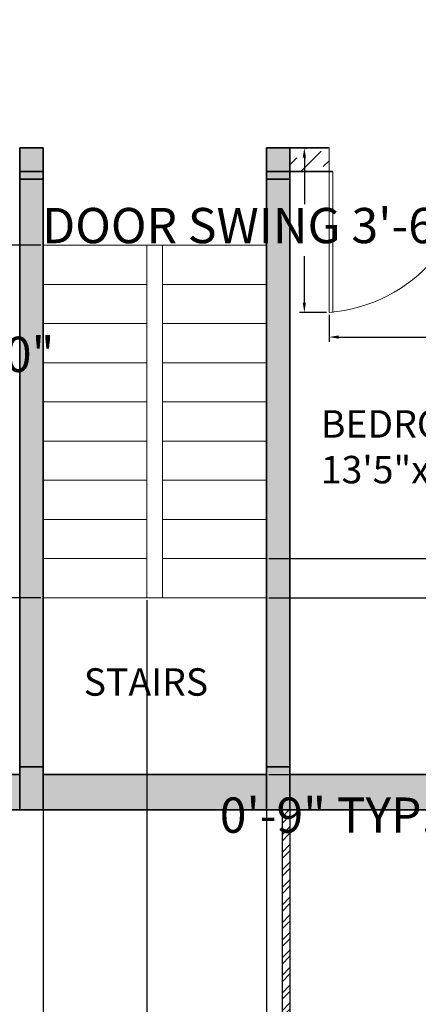
# Model space of a CAD drawing. Units: inches. Extents: x 9689 to 10369, y 10965 to 11626.
# Tile 4 of 11: x 10005 to 10107, y 11108 to 11359. Entities that reach past the tile are written whole.
import ezdxf

# ---------------------------------------------------------------- set-up
doc = ezdxf.new("R2010")
doc.units = ezdxf.units.IN
for name, color, linetype, lineweight in [('A-ANNO-DIMS', 2, 'Continuous', 18), ('A-AREA-IDEN', 7, 'Continuous', 18), ('A-COLS', 7, 'Continuous', 35), ('A-DOOR', 4, 'Continuous', 18), ('A-FLOR', 7, 'Continuous', 25), ('A-FLOR-PATT', 252, 'Continuous', 13), ('A-FLOR-STRS', 7, 'Continuous', 18), ('A-WALL', 7, 'Continuous', 35), ('A-WALL-PATT', 252, 'Continuous', 13)]:
    doc.layers.add(name, color=color, linetype=linetype, lineweight=lineweight)
doc.layers.add('A-COLS-PATT', color=18, linetype='Continuous', lineweight=13, true_color=0x000000)
doc.styles.get("Standard").update_dxf_attribs({"font": 'arial.ttf'})
doc.dimstyles.new('ISO-25', dxfattribs={"dimtxt": 9, "dimasz": 2.5, "dimexe": 1.25, "dimexo": 0.625, "dimgap": 2, "dimtad": 0, "dimtih": 1, "dimtoh": 1, "dimdec": 1, "dimlunit": 4, "dimtxsty": 'Standard', "dimcen": 2.5, "dimadec": 0, "dimazin": 0, "dimtfac": 0.5, "dimtdec": 1, "dimtmove": 0, "dimatfit": 3, "dimfxl": 1, "dimarcsym": 0})

# ---------------------------------------------------------------- blocks, each defined once
blk = doc.blocks.new('DOOR-SWING-36')
for p, q in [((0, 6), (0, 42)), ((1, 6), (1, 42)), ((0, 6), (0, 0))]:
    blk.add_line(p, q)
blk.add_arc((-3, 3), 39.12, 355.6013, 85.6013)
blk = doc.blocks.new('*D32')
at = {"layer": 'A-ANNO-DIMS', "color": 0, "lineweight": -2, "transparency": 16777216}
for p, q in [((10083.43, 11326.63), (10076.51, 11326.63)), ((10077.76, 11324.13), (10077.76, 11312.29)), ((10077.76, 11287.13), (10077.76, 11298.97)), ((10083.43, 11284.63), (10076.51, 11284.63))]:
    blk.add_line(p, q, dxfattribs=at)
at = {"layer": 'A-ANNO-DIMS', "color": 0, "transparency": 16777216}
for points in [[(10077.34, 11324.13), (10078.17, 11324.13), (10077.76, 11326.63)], [(10077.34, 11287.13), (10078.17, 11287.13), (10077.76, 11284.63)]]:
    blk.add_solid(points, dxfattribs=at)
at = {"layer": 'Defpoints', "color": 0, "transparency": 16777216}
for p in [(10084.06, 11326.63), (10077.76, 11284.63), (10084.06, 11284.63)]:
    blk.add_point(p, dxfattribs=at)
at = {"layer": 'A-ANNO-DIMS', "color": 0, "transparency": 16777216, "insert": (10077.76, 11305.63), "char_height": 9, "attachment_point": 5}
blk.add_mtext('DOOR SWING 3\'-6" TYP.', dxfattribs=at)
blk = doc.blocks.new('*D33')
at = {"layer": 'A-ANNO-DIMS', "color": 0, "lineweight": -2, "transparency": 16777216}
for p, q in [((10084.06, 11284.01), (10084.06, 11277.08)), ((10121.71, 11284.01), (10121.71, 11277.08)), ((10086.56, 11278.33), (10119.21, 11278.33)), ((10121.71, 11278.33), (10124.21, 11278.33))]:
    blk.add_line(p, q, dxfattribs=at)
at = {"layer": 'A-ANNO-DIMS', "color": 0, "transparency": 16777216}
for points in [[(10086.56, 11278.75), (10086.56, 11277.91), (10084.06, 11278.33)], [(10119.21, 11278.75), (10119.21, 11277.91), (10121.71, 11278.33)]]:
    blk.add_solid(points, dxfattribs=at)
at = {"layer": 'Defpoints', "color": 0, "transparency": 16777216}
for p in [(10084.06, 11284.63), (10121.71, 11284.63), (10121.71, 11278.33)]:
    blk.add_point(p, dxfattribs=at)
at = {"layer": 'A-ANNO-DIMS', "color": 0, "transparency": 16777216, "insert": (10164.13, 11278.33), "char_height": 9, "attachment_point": 5}
blk.add_mtext('3\'-1 1/2" TYP.', dxfattribs=at)
blk = doc.blocks.new('*D41')
at = {"layer": 'A-ANNO-DIMS', "color": 0, "lineweight": -2, "transparency": 16777216}
for p, q in [((10123.93, 11166.63), (10114.31, 11166.63)), ((10115.56, 11164.13), (10115.56, 11160.13)), ((10123.93, 11157.63), (10114.31, 11157.63)), ((10115.56, 11157.63), (10115.56, 11155.13)), ((10115.56, 11155.13), (10113.06, 11155.13))]:
    blk.add_line(p, q, dxfattribs=at)
at = {"layer": 'A-ANNO-DIMS', "color": 0, "transparency": 16777216}
for points in [[(10115.14, 11164.13), (10115.97, 11164.13), (10115.56, 11166.63)], [(10115.14, 11160.13), (10115.97, 11160.13), (10115.56, 11157.63)]]:
    blk.add_solid(points, dxfattribs=at)
at = {"layer": 'Defpoints', "color": 0, "transparency": 16777216}
for p in [(10124.56, 11166.63), (10115.56, 11157.63), (10124.56, 11157.63)]:
    blk.add_point(p, dxfattribs=at)
at = {"layer": 'A-ANNO-DIMS', "color": 0, "transparency": 16777216, "insert": (10083.63, 11155.13), "char_height": 9, "attachment_point": 5}
blk.add_mtext('0\'-9" TYP.', dxfattribs=at)
blk = doc.blocks.new('*D56')
at = {"layer": 'A-ANNO-DIMS', "color": 0, "lineweight": -2, "transparency": 16777216}
for p, q in [((9858.07, 11281.13), (9858.07, 11271.5)), ((9918.07, 11281.13), (9918.07, 11271.5)), ((9860.57, 11272.75), (9915.57, 11272.75)), ((9918.07, 11272.75), (9920.57, 11272.75))]:
    blk.add_line(p, q, dxfattribs=at)
at = {"layer": 'A-ANNO-DIMS', "color": 0, "transparency": 16777216}
for points in [[(9860.57, 11273.17), (9860.57, 11272.33), (9858.07, 11272.75)], [(9915.57, 11273.17), (9915.57, 11272.33), (9918.07, 11272.75)]]:
    blk.add_solid(points, dxfattribs=at)
at = {"layer": 'Defpoints', "color": 0, "transparency": 16777216}
for p in [(9858.07, 11281.75), (9918.07, 11281.75), (9918.07, 11272.75)]:
    blk.add_point(p, dxfattribs=at)
at = {"layer": 'A-ANNO-DIMS', "color": 0, "transparency": 16777216, "insert": (9969.27, 11272.75), "char_height": 9, "attachment_point": 5}
blk.add_mtext('LOVESEAT 5\'-0"', dxfattribs=at)
blk = doc.blocks.new('*D70')
at = {"layer": 'A-ANNO-DIMS', "color": 0, "lineweight": -2, "transparency": 16777216}
for p, q in [((10011.06, 11166.01), (10011.06, 10977.48)), ((10068.06, 11166.01), (10068.06, 10977.48)), ((10013.56, 10978.73), (10025.41, 10978.73)), ((10065.56, 10978.73), (10053.7, 10978.73))]:
    blk.add_line(p, q, dxfattribs=at)
at = {"layer": 'A-ANNO-DIMS', "color": 0, "transparency": 16777216}
for points in [[(10013.56, 10979.15), (10013.56, 10978.31), (10011.06, 10978.73)], [(10065.56, 10979.15), (10065.56, 10978.31), (10068.06, 10978.73)]]:
    blk.add_solid(points, dxfattribs=at)
at = {"layer": 'Defpoints', "color": 0, "transparency": 16777216}
for p in [(10011.06, 11166.63), (10068.06, 11166.63), (10068.06, 10978.73)]:
    blk.add_point(p, dxfattribs=at)
at = {"layer": 'A-ANNO-DIMS', "color": 0, "transparency": 16777216, "insert": (10039.56, 10978.73), "char_height": 9, "attachment_point": 5}
blk.add_mtext('4\'-9"', dxfattribs=at)
blk = doc.blocks.new('*D71')
at = {"layer": 'A-ANNO-DIMS', "color": 0, "lineweight": -2, "transparency": 16777216}
for p, q in [((10068.06, 11166.01), (10068.06, 10977.48)), ((10074.06, 11166.01), (10074.06, 10977.48)), ((10065.56, 10978.73), (10063.06, 10978.73)), ((10068.06, 10978.73), (10074.06, 10978.73)), ((10076.56, 10978.73), (10079.06, 10978.73))]:
    blk.add_line(p, q, dxfattribs=at)
at = {"layer": 'A-ANNO-DIMS', "color": 0, "transparency": 16777216}
for points in [[(10065.56, 10979.15), (10065.56, 10978.31), (10068.06, 10978.73)], [(10076.56, 10979.15), (10076.56, 10978.31), (10074.06, 10978.73)]]:
    blk.add_solid(points, dxfattribs=at)
at = {"layer": 'Defpoints', "color": 0, "transparency": 16777216}
for p in [(10068.06, 11166.63), (10074.06, 11166.63), (10074.06, 10978.73)]:
    blk.add_point(p, dxfattribs=at)
at = {"layer": 'A-ANNO-DIMS', "color": 0, "transparency": 16777216, "insert": (10093.02, 10978.73), "char_height": 9, "attachment_point": 5}
blk.add_mtext('0\'-6"', dxfattribs=at)
blk = doc.blocks.new('*D72')
at = {"layer": 'A-ANNO-DIMS', "color": 0, "lineweight": -2, "transparency": 16777216}
for p, q in [((10011.06, 11211.16), (10011.06, 10977.48)), ((10037.56, 11211.16), (10037.56, 10977.48)), ((10013.56, 10978.73), (10035.06, 10978.73)), ((10037.56, 10978.73), (10040.06, 10978.73))]:
    blk.add_line(p, q, dxfattribs=at)
at = {"layer": 'A-ANNO-DIMS', "color": 0, "transparency": 16777216}
for points in [[(10013.56, 10979.15), (10013.56, 10978.31), (10011.06, 10978.73)], [(10035.06, 10979.15), (10035.06, 10978.31), (10037.56, 10978.73)]]:
    blk.add_solid(points, dxfattribs=at)
at = {"layer": 'Defpoints', "color": 0, "transparency": 16777216}
for p in [(10011.06, 11211.79), (10037.56, 11211.79), (10037.56, 10978.73)]:
    blk.add_point(p, dxfattribs=at)
at = {"layer": 'A-ANNO-DIMS', "color": 0, "transparency": 16777216, "insert": (10064.58, 10978.73), "char_height": 9, "attachment_point": 5}
blk.add_mtext('2\'-2 1/2"', dxfattribs=at)
blk = doc.blocks.new('*D73')
at = {"layer": 'A-ANNO-DIMS', "color": 0, "lineweight": -2, "transparency": 16777216}
for p, q in [((10010.43, 11301.79), (9758.91, 11301.79)), ((9760.16, 11299.29), (9760.16, 11263.38)), ((9760.16, 11214.29), (9760.16, 11250.19)), ((10010.43, 11211.79), (9758.91, 11211.79))]:
    blk.add_line(p, q, dxfattribs=at)
at = {"layer": 'A-ANNO-DIMS', "color": 0, "transparency": 16777216}
for points in [[(9759.74, 11299.29), (9760.57, 11299.29), (9760.16, 11301.79)], [(9759.74, 11214.29), (9760.57, 11214.29), (9760.16, 11211.79)]]:
    blk.add_solid(points, dxfattribs=at)
at = {"layer": 'Defpoints', "color": 0, "transparency": 16777216}
for p in [(9760.16, 11301.79), (10011.06, 11301.79), (10011.06, 11211.79)]:
    blk.add_point(p, dxfattribs=at)
at = {"layer": 'A-ANNO-DIMS', "color": 0, "transparency": 16777216, "insert": (9760.16, 11256.79), "char_height": 9, "attachment_point": 5}
blk.add_mtext('7\'-6"', dxfattribs=at)
blk = doc.blocks.new('*D74')
at = {"layer": 'A-ANNO-DIMS', "color": 0, "lineweight": -2, "transparency": 16777216}
for p, q in [((10285.96, 11221.79), (10285.96, 11224.29)), ((10285.96, 11224.29), (10288.46, 11224.29)), ((10068.68, 11221.79), (10287.21, 11221.79)), ((10285.96, 11214.29), (10285.96, 11219.29)), ((10068.68, 11211.79), (10287.21, 11211.79))]:
    blk.add_line(p, q, dxfattribs=at)
at = {"layer": 'A-ANNO-DIMS', "color": 0, "transparency": 16777216}
for points in [[(10285.54, 11219.29), (10286.37, 11219.29), (10285.96, 11221.79)], [(10285.54, 11214.29), (10286.37, 11214.29), (10285.96, 11211.79)]]:
    blk.add_solid(points, dxfattribs=at)
at = {"layer": 'Defpoints', "color": 0, "transparency": 16777216}
for p in [(10068.06, 11221.79), (10285.96, 11221.79), (10068.06, 11211.79)]:
    blk.add_point(p, dxfattribs=at)
at = {"layer": 'A-ANNO-DIMS', "color": 0, "transparency": 16777216, "insert": (10305.92, 11224.29), "char_height": 9, "attachment_point": 5}
blk.add_mtext('0\'-10"', dxfattribs=at)
blk = doc.blocks.new('*D75')
at = {"layer": 'A-ANNO-DIMS', "color": 0, "lineweight": -2, "transparency": 16777216}
for p, q in [((10068.68, 11211.79), (10287.21, 11211.79)), ((10285.96, 11209.29), (10285.96, 11195.81)), ((10285.96, 11169.13), (10285.96, 11182.61)), ((10068.68, 11166.63), (10287.21, 11166.63))]:
    blk.add_line(p, q, dxfattribs=at)
at = {"layer": 'A-ANNO-DIMS', "color": 0, "transparency": 16777216}
for points in [[(10285.54, 11209.29), (10286.37, 11209.29), (10285.96, 11211.79)], [(10285.54, 11169.13), (10286.37, 11169.13), (10285.96, 11166.63)]]:
    blk.add_solid(points, dxfattribs=at)
at = {"layer": 'Defpoints', "color": 0, "transparency": 16777216}
for p in [(10068.06, 11211.79), (10285.96, 11211.79), (10068.06, 11166.63)]:
    blk.add_point(p, dxfattribs=at)
at = {"layer": 'A-ANNO-DIMS', "color": 0, "transparency": 16777216, "insert": (10285.96, 11189.21), "char_height": 9, "attachment_point": 5}
blk.add_mtext('3\'-9"', dxfattribs=at)

msp = doc.modelspace()

# ---------------------------------------------------------------- hatches: boundary and pattern name
at = {"layer": 'A-COLS-PATT'}
h = msp.add_hatch(color=256, dxfattribs=at)
h.dxf.hatch_style = 1
h.paths.add_polyline_path([(10011.06, 11326.63), (10005.06, 11326.63), (10005.06, 11320.63), (10005.06, 11318.63), (10011.06, 11318.63), (10011.06, 11320.63)])
h = msp.add_hatch(color=256, dxfattribs=at)
h.dxf.hatch_style = 1
h.paths.add_polyline_path([(10074.06, 11326.63), (10068.06, 11326.63), (10068.06, 11320.63), (10068.06, 11318.63), (10074.06, 11318.63), (10074.06, 11320.63)])
h = msp.add_hatch(color=256, dxfattribs=at)
h.dxf.hatch_style = 1
h.paths.add_polyline_path([(10011.06, 11166.63), (10011.06, 11168.63), (10005.06, 11168.63), (10005.06, 11166.63), (10005.06, 11157.63), (10011.06, 11157.63)])
h = msp.add_hatch(color=256, dxfattribs=at)
h.dxf.hatch_style = 1
h.paths.add_polyline_path([(10074.06, 11166.63), (10074.06, 11168.63), (10068.06, 11168.63), (10068.06, 11166.63), (10068.06, 11157.63), (10074.06, 11157.63)])
at = {"layer": 'A-FLOR-PATT'}
h = msp.add_hatch(dxfattribs=at)
h.set_pattern_fill('STEEL', color=256)
h.set_pattern_definition([(45, (0, 0), (-2.245064, 2.245064), []), (45, (0, 1.5875), (-2.245064, 2.245064), [])])
h.paths.add_polyline_path([(10074.06, 11157.63), (10072.06, 11157.63), (10072.06, 11077.63), (9985.06, 11077.63), (9985.06, 11075.63), (10074.06, 11075.63)])
h.paths.add_polyline_path([(9907.06, 11157.63), (9905.06, 11157.63), (9905.06, 11075.63), (9937.06, 11075.63), (9937.06, 11077.63), (9907.06, 11077.63)])
at = {"layer": 'A-WALL-PATT'}
h = msp.add_hatch(dxfattribs=at)
h.set_pattern_fill('ANSI33', color=256)
h.paths.add_polyline_path([(9843.06, 11538.63), (9811.06, 11538.63), (9811.06, 11529.63), (9843.06, 11529.63)])
h.paths.add_polyline_path([(9923.06, 11538.63), (9891.06, 11538.63), (9891.06, 11529.63), (9923.06, 11529.63)])
h.paths.add_polyline_path([(9929.06, 11527.63), (9923.06, 11527.63), (9923.06, 11380.63), (9929.06, 11380.63)])
h.paths.add_polyline_path([(9939.06, 11538.63), (9929.06, 11538.63), (9929.06, 11529.63), (9939.06, 11529.63, -0.071068)])
h.paths.add_polyline_path([(10035.06, 11538.63), (10013.06, 11538.63), (10013.06, 11529.63), (10022.06, 11529.63), (10022.06, 11507.38), (10022.06, 11502.38), (10022.06, 11482.38), (10022.06, 11478.38), (10022.06, 11456.13, -0.038405), (10026.06, 11456.13), (10026.06, 11502.38), (10026.06, 11529.63), (10035.06, 11529.63)])
h.paths.add_polyline_path([(10068.06, 11538.63), (10059.06, 11538.63), (10059.06, 11529.63), (10068.06, 11529.63)])
h.paths.add_polyline_path([(10074.06, 11527.63), (10068.06, 11527.63), (10068.06, 11431.13), (10026.06, 11431.13), (10022.06, 11431.13), (9980.06, 11431.13), (9976.06, 11431.13), (9976.06, 11425.13), (10068.06, 11425.13), (10068.06, 11380.63), (10074.06, 11380.63)])
h.paths.add_polyline_path([(10124.56, 11538.63), (10074.06, 11538.63), (10074.06, 11529.63), (10124.56, 11529.63)])
h.paths.add_polyline_path([(9980.06, 11507.38), (9980.06, 11529.63), (9989.06, 11529.63), (9989.06, 11538.63), (9976.06, 11538.63), (9976.06, 11529.63), (9976.06, 11503.38), (9976.06, 11483.38), (9976.06, 11478.38), (9980.06, 11478.38), (9997.06, 11478.38, -0.038405), (9997.06, 11482.38), (9980.06, 11482.38)])
h.paths.add_polyline_path([(10235.06, 11538.63), (10184.56, 11538.63), (10184.56, 11529.63), (10235.06, 11529.63)])
h.paths.add_polyline_path([(10244.06, 11527.63), (10235.06, 11527.63), (10235.06, 11485.13), (10244.06, 11485.13)])
h.paths.add_polyline_path([(10244.06, 11425.13), (10235.06, 11425.13), (10235.06, 11380.63), (10244.06, 11380.63)])
h.paths.add_polyline_path([(10233.06, 11380.63), (10120.06, 11380.63, -0.038405), (10120.06, 11374.63), (10133.04, 11374.63), (10133.04, 11326.63), (10120.06, 11326.63, -0.038405), (10120.06, 11320.63), (10149.19, 11320.63), (10149.19, 11326.63), (10136.04, 11326.63), (10136.04, 11374.63), (10233.06, 11374.63)])
h.paths.add_polyline_path([(10084.06, 11380.63), (10076.06, 11380.63), (10076.06, 11374.63), (10084.06, 11374.63)])
h.paths.add_polyline_path([(10244.06, 11374.63), (10235.06, 11374.63), (10235.06, 11362.63), (10244.06, 11362.63)])
h.paths.add_polyline_path([(10244.06, 11338.63), (10235.06, 11338.63), (10235.06, 11326.63), (10244.06, 11326.63)])
h.paths.add_polyline_path([(10233.06, 11326.63), (10173.19, 11326.63, -0.055385), (10173.19, 11320.63), (10233.06, 11320.63)], flags=0)
h.paths.add_polyline_path([(10244.06, 11320.63), (10235.06, 11320.63), (10235.06, 11273.63), (10244.06, 11273.63)])
h = msp.add_hatch(dxfattribs=at)
h.set_pattern_fill('ANSI36', color=256)
h.paths.add_polyline_path([(10233.06, 11326.63), (10173.19, 11326.63, -0.055385), (10173.19, 11320.63), (10233.06, 11320.63)])
h.paths.add_polyline_path([(10244.06, 11213.63), (10235.06, 11213.63), (10235.06, 11166.63), (10244.06, 11166.63)])
h.paths.add_polyline_path([(10233.06, 11166.63), (10184.56, 11166.63), (10184.56, 11157.63), (10233.06, 11157.63)])
h.paths.add_polyline_path([(10124.56, 11166.63), (10074.06, 11166.63), (10074.06, 11157.63), (10124.56, 11157.63)])
h.paths.add_polyline_path([(10074.06, 11318.63), (10068.06, 11318.63), (10068.06, 11168.63), (10074.06, 11168.63)])
h.paths.add_polyline_path([(10068.06, 11166.63), (10011.06, 11166.63), (10011.06, 11157.63), (10068.06, 11157.63)])
h.paths.add_polyline_path([(10011.06, 11318.63), (10005.06, 11318.63), (10005.06, 11168.63), (10011.06, 11168.63)])
h.paths.add_polyline_path([(10005.06, 11166.63), (9985.06, 11166.63), (9985.06, 11157.63), (10005.06, 11157.63)])
h.paths.add_polyline_path([(9937.06, 11166.63), (9898.06, 11166.63), (9898.06, 11157.63), (9937.06, 11157.63, -0.042779)])
h.paths.add_polyline_path([(9850.06, 11166.63), (9813.06, 11166.63), (9813.06, 11157.63), (9850.06, 11157.63)])
h.paths.add_polyline_path([(9811.06, 11213.63), (9802.06, 11213.63), (9802.06, 11166.63), (9811.06, 11166.63)])
h.paths.add_polyline_path([(9811.06, 11320.63), (9802.06, 11320.63), (9802.06, 11273.63), (9811.06, 11273.63)])
h.paths.add_polyline_path([(9811.06, 11439.11), (9802.06, 11439.11), (9802.06, 11326.63), (9811.06, 11326.63)])
h.paths.add_polyline_path([(9957.06, 11326.63), (9813.06, 11326.63), (9813.06, 11320.63), (9957.06, 11320.63)])
h.paths.add_polyline_path([(9811.06, 11527.63), (9802.06, 11527.63), (9802.06, 11499.11), (9811.06, 11499.11)])
h = msp.add_hatch(dxfattribs=at)
h.set_pattern_fill('ANSI36', color=256)
h.paths.add_polyline_path([(10084.06, 11326.63), (10074.06, 11326.63), (10074.06, 11320.63), (10084.06, 11320.63)])

# ---------------------------------------------------------------- linework, layer by layer
at = {"layer": 'A-COLS'}
for p, q in [((10005.06, 11320.63), (10005.06, 11326.63)), ((10005.06, 11326.63), (10011.06, 11326.63)), ((10005.06, 11326.63), (10011.06, 11326.63)), ((10011.06, 11320.63), (10011.06, 11326.63)), ((10068.06, 11320.63), (10068.06, 11326.63)), ((10074.06, 11320.63), (10074.06, 11326.63)), ((10005.06, 11320.63), (10011.06, 11320.63)), ((10011.06, 11318.63), (10005.06, 11318.63)), ((10074.06, 11318.63), (10068.06, 11318.63)), ((10005.06, 11168.63), (10011.06, 11168.63)), ((10068.06, 11168.63), (10074.06, 11168.63)), ((10005.06, 11166.63), (10005.06, 11157.63)), ((10011.06, 11166.63), (10011.06, 11157.63)), ((10068.06, 11166.63), (10068.06, 11157.63)), ((10074.06, 11166.63), (10074.06, 11157.63))]:
    msp.add_line(p, q, dxfattribs=at)
at = {"layer": 'A-DOOR'}
msp.add_line((10084.06, 11320.63), (10085.06, 11320.63), dxfattribs=at)
at = {"layer": 'A-FLOR'}
for p, q in [((10072.06, 11157.63), (10072.06, 11077.63)), ((10074.06, 11157.63), (10074.06, 11075.63))]:
    msp.add_line(p, q, dxfattribs=at)
at = {"layer": 'A-FLOR-STRS'}
for p, q in [((10011.06, 11301.79), (10068.06, 11301.79)), ((10037.56, 11211.79), (10037.56, 11301.79)), ((10041.56, 11211.79), (10041.56, 11301.79)), ((10011.06, 11291.79), (10037.56, 11291.79)), ((10041.56, 11291.79), (10068.06, 11291.79)), ((10011.06, 11281.79), (10037.56, 11281.79)), ((10041.56, 11281.79), (10068.06, 11281.79)), ((10011.06, 11271.79), (10037.56, 11271.79)), ((10041.56, 11271.79), (10068.06, 11271.79)), ((10011.06, 11261.79), (10037.56, 11261.79)), ((10041.56, 11261.79), (10068.06, 11261.79)), ((10011.06, 11251.79), (10037.56, 11251.79)), ((10041.56, 11251.79), (10068.06, 11251.79)), ((10011.06, 11241.79), (10037.56, 11241.79)), ((10041.56, 11241.79), (10068.06, 11241.79)), ((10011.06, 11231.79), (10037.56, 11231.79)), ((10041.56, 11231.79), (10068.06, 11231.79)), ((10011.06, 11221.79), (10037.56, 11221.79)), ((10041.56, 11221.79), (10068.06, 11221.79)), ((10011.06, 11211.79), (10068.06, 11211.79))]:
    msp.add_line(p, q, dxfattribs=at)
at = {"layer": 'A-WALL'}
for p, q in [((10068.06, 11326.63), (10084.06, 11326.63)), ((10068.06, 11326.63), (10084.06, 11326.63)), ((10074.06, 11326.63), (10084.06, 11326.63)), ((10005.06, 11166.63), (10005.06, 11320.63)), ((10011.06, 11166.63), (10011.06, 11320.63)), ((10068.06, 11320.63), (10068.06, 11166.63)), ((10068.06, 11320.63), (10085.06, 11320.63)), ((10074.06, 11320.63), (10074.06, 11166.63)), ((10074.06, 11320.63), (10084.06, 11320.63)), ((10005.06, 11166.63), (9984.06, 11166.63)), ((10068.06, 11166.63), (10011.06, 11166.63)), ((10235.06, 11166.63), (10074.06, 11166.63)), ((10244.06, 11157.63), (9985.06, 11157.63))]:
    msp.add_line(p, q, dxfattribs=at)

# ---------------------------------------------------------------- block references
at = {"layer": 'A-DOOR', "extrusion": (0, 0, -1), "zscale": -1, "rotation": 180}
msp.add_blockref('DOOR-SWING-36', (-10084.06, 11326.63), dxfattribs=at)

# ---------------------------------------------------------------- texts
at = {"layer": 'A-AREA-IDEN', "char_height": 7, "attachment_point": 1}
for s, width, insert in [('{\\fArial|b1|i0|c0|p34;BEDROOM\\P13\'5"x12\'6"}', 73.0838, (10081.97, 11259.66)), ('{\\fArial|b1|i0|c0|p34;STAIRS}', 46.8133, (10021.41, 11193.78))]:
    msp.add_mtext_dynamic_manual_height_columns(s, width=width, gutter_width=12.5, heights=[0], dxfattribs=dict(at, insert=insert))

# ---------------------------------------------------------------- dimensions: what is measured, and where the dimension line sits
at = {"layer": 'A-ANNO-DIMS'}
for base, p1, p2, text, picture, middle in [((10077.76, 11284.63), (10084.06, 11326.63), (10084.06, 11284.63), 'DOOR SWING <> TYP.', '*D32', (10077.76, 11305.63)), ((10115.56, 11157.63), (10124.56, 11166.63), (10124.56, 11157.63), '<> TYP.', '*D41', (10083.63, 11155.13))]:
    dim = msp.add_linear_dim(base=base, p1=p1, p2=p2, angle=270, text=text, dimstyle='ISO-25', override={"dimdec": 1, "dimlfac": 1, "dimrnd": 0, "dimzin": 1, "dimdsep": 46, "dimlunit": 4, "dimfrac": 2}, dxfattribs=at)
    dim.commit()
    dim.dimension.update_dxf_attribs({"geometry": picture, "text_midpoint": middle})
for base, p1, p2, picture, middle in [((9760.16, 11301.79), (10011.06, 11211.79), (10011.06, 11301.79), '*D73', (9760.16, 11256.79)), ((10285.96, 11221.79), (10068.06, 11211.79), (10068.06, 11221.79), '*D74', (10305.92, 11224.29)), ((10285.96, 11211.79), (10068.06, 11166.63), (10068.06, 11211.79), '*D75', (10285.96, 11189.21))]:
    dim = msp.add_linear_dim(base=base, p1=p1, p2=p2, angle=90, dimstyle='ISO-25', override={"dimdec": 1, "dimlfac": 1, "dimrnd": 0, "dimzin": 1, "dimdsep": 46, "dimlunit": 4, "dimfrac": 2}, dxfattribs=at)
    dim.commit()
    dim.dimension.update_dxf_attribs({"geometry": picture, "text_midpoint": middle})
for base, p1, p2, text, picture, middle in [((10121.7136, 11278.3301), (10084.0568, 11284.6301), (10121.7136, 11284.6301), '<> TYP.', '*D33', (10164.126, 11278.3301)), ((9918.07, 11272.75), (9858.07, 11281.75), (9918.07, 11281.75), 'LOVESEAT <>', '*D56', (9969.27, 11272.75))]:
    dim = msp.add_linear_dim(base=base, p1=p1, p2=p2, text=text, dimstyle='ISO-25', override={"dimdec": 1, "dimlfac": 1, "dimrnd": 0, "dimzin": 1, "dimdsep": 46, "dimlunit": 4, "dimfrac": 2}, dxfattribs=at)
    dim.commit()
    dim.dimension.update_dxf_attribs({"geometry": picture, "text_midpoint": middle})
for base, p1, p2, picture, middle in [((10037.56, 10978.73), (10011.06, 11211.79), (10037.56, 11211.79), '*D72', (10064.58, 10978.73)), ((10068.06, 10978.73), (10011.06, 11166.63), (10068.06, 11166.63), '*D70', (10039.56, 10978.73)), ((10074.06, 10978.73), (10068.06, 11166.63), (10074.06, 11166.63), '*D71', (10093.02, 10978.73))]:
    dim = msp.add_linear_dim(base=base, p1=p1, p2=p2, dimstyle='ISO-25', override={"dimdec": 1, "dimlfac": 1, "dimrnd": 0, "dimzin": 1, "dimdsep": 46, "dimlunit": 4, "dimfrac": 2}, dxfattribs=at)
    dim.commit()
    dim.dimension.update_dxf_attribs({"geometry": picture, "text_midpoint": middle})

doc.saveas('drawing.dxf')
